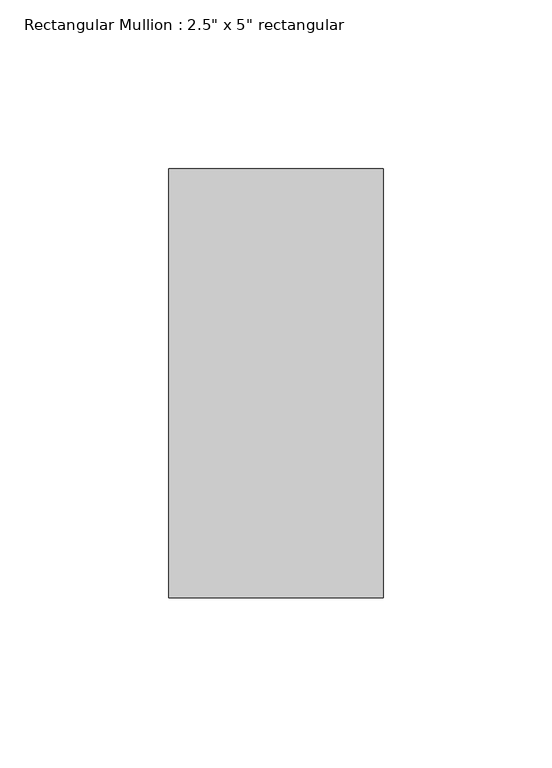
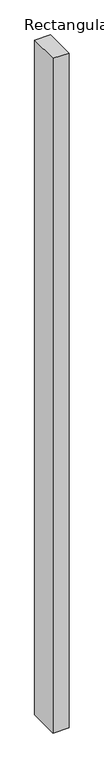
"""IFC4 building model written with IfcOpenShell, lengths in millimetres: member geometry."""

from ifc_helpers import new_model, si_unit, frame, origin, place, context, project, spatial, polyline, outline, extrude, source, transform, mapped, element, save


def member_2680e53c(model_context):
    return source(origin(), model_context, "Body", "SweptSolid", [
        extrude(outline(polyline([(0.0, 63.5), (0.0, -63.5), (-63.5, -63.5), (-63.5, 63.5), (0.0, 63.5)])), frame((0.0, 0.0, -2846.788773), z_axis=(0.0, 0.0, 1.0), x_axis=(1.0, 0.0, 0.0)), (0.0, 0.0, 1.0), 2846.788773),
    ])


if __name__ == "__main__":
    model = new_model("IFC4")
    model_context = context("Model", 3, world=origin())
    ifc_project = project(units=[si_unit("LENGTHUNIT", "METRE", prefix="MILLI")], contexts=[model_context])
    site = spatial("IfcSite", under=ifc_project)
    building = spatial("IfcBuilding", under=site)
    placement = place(None, origin())
    member_shape = member_2680e53c(model_context)
    element("IfcMember", 1, ObjectType="Rectangular Mullion : 2.5\" x 5\" rectangular", at=placement, inside=building, context=model_context, shape_type="MappedRepresentation", body=[
        mapped(member_shape, transform((0.0, 0.0, 0.0), x_axis=(1.0, 0.0, 0.0), y_axis=(0.0, 1.0, 0.0), z_axis=(0.0, 0.0, 1.0))),
    ])
    save(model, "model.ifc")

# Revit data of these elements
# Type "Rectangular Mullion : 2.5\" x 5\" rectangular"
#   built-in parameter 1007304 = 0.416667 (stored number, unit not read)
#   built-in parameter 1007301 = 0.104167 (stored number, unit not read)
#   built-in parameter 1007300 = 0.104167 (stored number, unit not read)
# Element 1 (IfcMember, "Rectangular Mullion : 2.5\" x 5\" rectangular")
#   Materials on its faces: "Aluminum"
# Materials
#   "Aluminum": class "Metal", colour RGB 247 247 247, transparency 0, Description = "Aluminum 6061", Cost = 0
